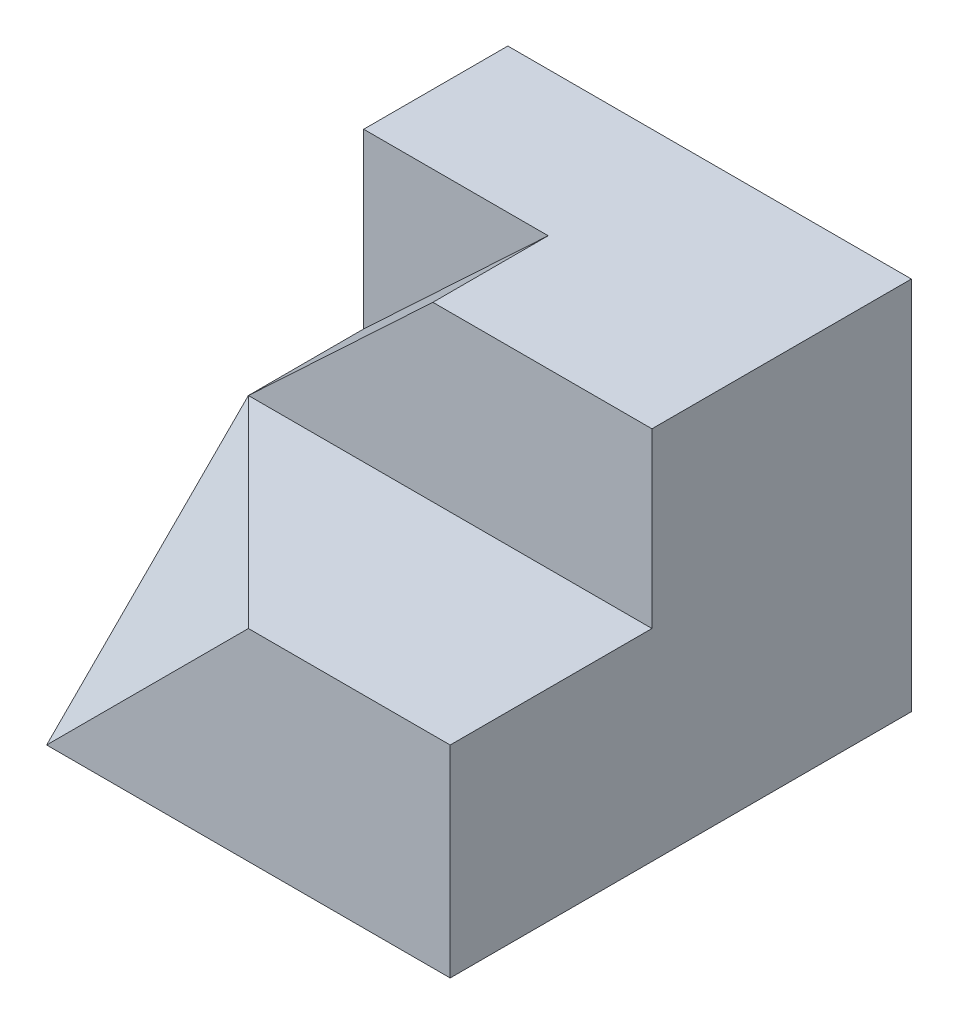
ISO-10303-21;
HEADER;
FILE_DESCRIPTION(('STEP AP214'),'2;1');
FILE_NAME('part.step','',(''),(''),'','','');
FILE_SCHEMA(('AUTOMOTIVE_DESIGN { 1 0 10303 214 1 1 1 1 }'));
ENDSEC;
DATA;
#1=APPLICATION_CONTEXT('core data for automotive mechanical design processes');
#2=APPLICATION_PROTOCOL_DEFINITION('international standard','automotive_design',2000,#1);
#3=PRODUCT_CONTEXT('',#1,'mechanical');
#4=PRODUCT('Part','Part','',(#3));
#5=PRODUCT_RELATED_PRODUCT_CATEGORY('part','',(#4));
#6=PRODUCT_DEFINITION_FORMATION('','',#4);
#7=PRODUCT_DEFINITION_CONTEXT('part definition',#1,'design');
#8=PRODUCT_DEFINITION('design','',#6,#7);
#9=PRODUCT_DEFINITION_SHAPE('','',#8);
#10=(LENGTH_UNIT() NAMED_UNIT(*) SI_UNIT(.MILLI.,.METRE.));
#11=(NAMED_UNIT(*) PLANE_ANGLE_UNIT() SI_UNIT($,.RADIAN.));
#12=(NAMED_UNIT(*) SI_UNIT($,.STERADIAN.) SOLID_ANGLE_UNIT());
#13=UNCERTAINTY_MEASURE_WITH_UNIT(LENGTH_MEASURE(1.E-05),#10,'distance_accuracy_value','');
#14=(GEOMETRIC_REPRESENTATION_CONTEXT(3) GLOBAL_UNCERTAINTY_ASSIGNED_CONTEXT((#13)) GLOBAL_UNIT_ASSIGNED_CONTEXT((#10,
#11,#12)) REPRESENTATION_CONTEXT('',''));
#15=CARTESIAN_POINT('',(0.,0.,0.));
#16=DIRECTION('',(0.,0.,1.));
#17=DIRECTION('',(1.,0.,0.));
#18=AXIS2_PLACEMENT_3D('',#15,#16,#17);
#19=CARTESIAN_POINT('',(0.,65.,40.));
#20=DIRECTION('',(1.,0.,0.));
#21=DIRECTION('',(0.,0.,-1.));
#22=AXIS2_PLACEMENT_3D('',#19,#20,#21);
#23=PLANE('',#22);
#24=DIRECTION('',(0.,0.707106781186548,-0.707106781186548));
#25=VECTOR('',#24,1.);
#26=CARTESIAN_POINT('',(0.,35.,5.));
#27=LINE('',#26,#25);
#28=CARTESIAN_POINT('',(0.,0.,40.));
#29=VERTEX_POINT('',#28);
#30=CARTESIAN_POINT('',(0.,35.,5.));
#31=VERTEX_POINT('',#30);
#32=EDGE_CURVE('E132',#29,#31,#27,.T.);
#33=ORIENTED_EDGE('',*,*,#32,.T.);
#34=DIRECTION('',(0.,0.,1.));
#35=VECTOR('',#34,1.);
#36=CARTESIAN_POINT('',(0.,35.,-15.));
#37=LINE('',#36,#35);
#38=CARTESIAN_POINT('',(0.,35.,-15.));
#39=VERTEX_POINT('',#38);
#40=EDGE_CURVE('E249',#39,#31,#37,.T.);
#41=ORIENTED_EDGE('',*,*,#40,.F.);
#42=DIRECTION('',(0.,-1.,0.));
#43=VECTOR('',#42,1.);
#44=CARTESIAN_POINT('',(0.,65.,-15.));
#45=LINE('',#44,#43);
#46=CARTESIAN_POINT('',(0.,65.,-15.));
#47=VERTEX_POINT('',#46);
#48=EDGE_CURVE('E238',#47,#39,#45,.T.);
#49=ORIENTED_EDGE('',*,*,#48,.F.);
#50=DIRECTION('',(0.,0.,-1.));
#51=VECTOR('',#50,1.);
#52=CARTESIAN_POINT('',(0.,65.,40.));
#53=LINE('',#52,#51);
#54=CARTESIAN_POINT('',(0.,65.,-40.));
#55=VERTEX_POINT('',#54);
#56=EDGE_CURVE('E99',#47,#55,#53,.T.);
#57=ORIENTED_EDGE('',*,*,#56,.T.);
#58=DIRECTION('',(0.,-1.,0.));
#59=VECTOR('',#58,1.);
#60=CARTESIAN_POINT('',(0.,65.,-40.));
#61=LINE('',#60,#59);
#62=CARTESIAN_POINT('',(0.,0.,-40.));
#63=VERTEX_POINT('',#62);
#64=EDGE_CURVE('E115',#55,#63,#61,.T.);
#65=ORIENTED_EDGE('',*,*,#64,.T.);
#66=DIRECTION('',(0.,0.,-1.));
#67=VECTOR('',#66,1.);
#68=CARTESIAN_POINT('',(0.,0.,40.));
#69=LINE('',#68,#67);
#70=EDGE_CURVE('E11',#29,#63,#69,.T.);
#71=ORIENTED_EDGE('',*,*,#70,.F.);
#72=EDGE_LOOP('',(#33,#41,#49,#57,#65,#71));
#73=FACE_BOUND('',#72,.T.);
#74=ADVANCED_FACE('F44',(#73),#23,.F.);
#75=CARTESIAN_POINT('',(0.,0.,40.));
#76=DIRECTION('',(0.,0.,1.));
#77=DIRECTION('',(1.,0.,0.));
#78=AXIS2_PLACEMENT_3D('',#75,#76,#77);
#79=PLANE('',#78);
#80=DIRECTION('',(1.,0.,0.));
#81=VECTOR('',#80,1.);
#82=CARTESIAN_POINT('',(0.,35.,40.));
#83=LINE('',#82,#81);
#84=CARTESIAN_POINT('',(35.,35.,40.));
#85=VERTEX_POINT('',#84);
#86=CARTESIAN_POINT('',(70.,35.,40.));
#87=VERTEX_POINT('',#86);
#88=EDGE_CURVE('E254',#85,#87,#83,.T.);
#89=ORIENTED_EDGE('',*,*,#88,.F.);
#90=DIRECTION('',(-0.707106781186548,-0.707106781186548,0.));
#91=VECTOR('',#90,1.);
#92=CARTESIAN_POINT('',(0.,0.,40.));
#93=LINE('',#92,#91);
#94=EDGE_CURVE('E56',#85,#29,#93,.T.);
#95=ORIENTED_EDGE('',*,*,#94,.T.);
#96=DIRECTION('',(1.,0.,0.));
#97=VECTOR('',#96,1.);
#98=CARTESIAN_POINT('',(0.,0.,40.));
#99=LINE('',#98,#97);
#100=CARTESIAN_POINT('',(70.,0.,40.));
#101=VERTEX_POINT('',#100);
#102=EDGE_CURVE('E70',#29,#101,#99,.T.);
#103=ORIENTED_EDGE('',*,*,#102,.T.);
#104=DIRECTION('',(0.,1.,0.));
#105=VECTOR('',#104,1.);
#106=CARTESIAN_POINT('',(70.,0.,40.));
#107=LINE('',#106,#105);
#108=EDGE_CURVE('E111',#101,#87,#107,.T.);
#109=ORIENTED_EDGE('',*,*,#108,.T.);
#110=EDGE_LOOP('',(#89,#95,#103,#109));
#111=FACE_BOUND('',#110,.T.);
#112=ADVANCED_FACE('F135',(#111),#79,.T.);
#113=CARTESIAN_POINT('',(0.,35.,5.));
#114=DIRECTION('',(0.,-1.,0.));
#115=DIRECTION('',(0.,0.,-1.));
#116=AXIS2_PLACEMENT_3D('',#113,#114,#115);
#117=PLANE('',#116);
#118=DIRECTION('',(0.707106781186548,0.,0.707106781186548));
#119=VECTOR('',#118,1.);
#120=CARTESIAN_POINT('',(35.,35.,40.));
#121=LINE('',#120,#119);
#122=EDGE_CURVE('E276',#31,#85,#121,.T.);
#123=ORIENTED_EDGE('',*,*,#122,.T.);
#124=ORIENTED_EDGE('',*,*,#88,.T.);
#125=DIRECTION('',(0.,0.,1.));
#126=VECTOR('',#125,1.);
#127=CARTESIAN_POINT('',(70.,35.,5.));
#128=LINE('',#127,#126);
#129=CARTESIAN_POINT('',(70.,35.,5.));
#130=VERTEX_POINT('',#129);
#131=EDGE_CURVE('E122',#130,#87,#128,.T.);
#132=ORIENTED_EDGE('',*,*,#131,.F.);
#133=DIRECTION('',(1.,0.,0.));
#134=VECTOR('',#133,1.);
#135=CARTESIAN_POINT('',(0.,35.,5.));
#136=LINE('',#135,#134);
#137=EDGE_CURVE('E257',#31,#130,#136,.T.);
#138=ORIENTED_EDGE('',*,*,#137,.F.);
#139=EDGE_LOOP('',(#123,#124,#132,#138));
#140=FACE_BOUND('',#139,.T.);
#141=ADVANCED_FACE('F139',(#140),#117,.F.);
#142=CARTESIAN_POINT('',(70.,65.,40.));
#143=DIRECTION('',(0.,-1.,0.));
#144=DIRECTION('',(1.,0.,0.));
#145=AXIS2_PLACEMENT_3D('',#142,#143,#144);
#146=PLANE('',#145);
#147=DIRECTION('',(-1.,0.,0.));
#148=VECTOR('',#147,1.);
#149=CARTESIAN_POINT('',(32.,65.,-15.));
#150=LINE('',#149,#148);
#151=CARTESIAN_POINT('',(32.,65.,-15.));
#152=VERTEX_POINT('',#151);
#153=EDGE_CURVE('E245',#152,#47,#150,.T.);
#154=ORIENTED_EDGE('',*,*,#153,.F.);
#155=DIRECTION('',(0.,0.,1.));
#156=VECTOR('',#155,1.);
#157=CARTESIAN_POINT('',(32.,65.,-15.));
#158=LINE('',#157,#156);
#159=CARTESIAN_POINT('',(32.,65.,5.));
#160=VERTEX_POINT('',#159);
#161=EDGE_CURVE('E251',#152,#160,#158,.T.);
#162=ORIENTED_EDGE('',*,*,#161,.T.);
#163=DIRECTION('',(-1.,0.,0.));
#164=VECTOR('',#163,1.);
#165=CARTESIAN_POINT('',(70.,65.,5.));
#166=LINE('',#165,#164);
#167=CARTESIAN_POINT('',(70.,65.,5.));
#168=VERTEX_POINT('',#167);
#169=EDGE_CURVE('E100',#168,#160,#166,.T.);
#170=ORIENTED_EDGE('',*,*,#169,.F.);
#171=DIRECTION('',(0.,0.,-1.));
#172=VECTOR('',#171,1.);
#173=CARTESIAN_POINT('',(70.,65.,40.));
#174=LINE('',#173,#172);
#175=CARTESIAN_POINT('',(70.,65.,-40.));
#176=VERTEX_POINT('',#175);
#177=EDGE_CURVE('E87',#168,#176,#174,.T.);
#178=ORIENTED_EDGE('',*,*,#177,.T.);
#179=DIRECTION('',(-1.,0.,0.));
#180=VECTOR('',#179,1.);
#181=CARTESIAN_POINT('',(70.,65.,-40.));
#182=LINE('',#181,#180);
#183=EDGE_CURVE('E91',#176,#55,#182,.T.);
#184=ORIENTED_EDGE('',*,*,#183,.T.);
#185=ORIENTED_EDGE('',*,*,#56,.F.);
#186=EDGE_LOOP('',(#154,#162,#170,#178,#184,#185));
#187=FACE_BOUND('',#186,.T.);
#188=ADVANCED_FACE('F89',(#187),#146,.F.);
#189=CARTESIAN_POINT('',(0.,0.,40.));
#190=DIRECTION('',(0.,1.,0.));
#191=DIRECTION('',(0.,0.,1.));
#192=AXIS2_PLACEMENT_3D('',#189,#190,#191);
#193=PLANE('',#192);
#194=DIRECTION('',(1.,0.,0.));
#195=VECTOR('',#194,1.);
#196=CARTESIAN_POINT('',(0.,0.,-40.));
#197=LINE('',#196,#195);
#198=CARTESIAN_POINT('',(70.,0.,-40.));
#199=VERTEX_POINT('',#198);
#200=EDGE_CURVE('E107',#63,#199,#197,.T.);
#201=ORIENTED_EDGE('',*,*,#200,.T.);
#202=DIRECTION('',(0.,0.,-1.));
#203=VECTOR('',#202,1.);
#204=CARTESIAN_POINT('',(70.,0.,40.));
#205=LINE('',#204,#203);
#206=EDGE_CURVE('E55',#101,#199,#205,.T.);
#207=ORIENTED_EDGE('',*,*,#206,.F.);
#208=ORIENTED_EDGE('',*,*,#102,.F.);
#209=ORIENTED_EDGE('',*,*,#70,.T.);
#210=EDGE_LOOP('',(#201,#207,#208,#209));
#211=FACE_BOUND('',#210,.T.);
#212=ADVANCED_FACE('F127',(#211),#193,.F.);
#213=CARTESIAN_POINT('',(70.,0.,40.));
#214=DIRECTION('',(-1.,0.,0.));
#215=DIRECTION('',(0.,0.,1.));
#216=AXIS2_PLACEMENT_3D('',#213,#214,#215);
#217=PLANE('',#216);
#218=DIRECTION('',(0.,1.,0.));
#219=VECTOR('',#218,1.);
#220=CARTESIAN_POINT('',(70.,35.,5.));
#221=LINE('',#220,#219);
#222=EDGE_CURVE('E263',#130,#168,#221,.T.);
#223=ORIENTED_EDGE('',*,*,#222,.F.);
#224=ORIENTED_EDGE('',*,*,#131,.T.);
#225=ORIENTED_EDGE('',*,*,#108,.F.);
#226=ORIENTED_EDGE('',*,*,#206,.T.);
#227=DIRECTION('',(0.,1.,0.));
#228=VECTOR('',#227,1.);
#229=CARTESIAN_POINT('',(70.,0.,-40.));
#230=LINE('',#229,#228);
#231=EDGE_CURVE('E102',#199,#176,#230,.T.);
#232=ORIENTED_EDGE('',*,*,#231,.T.);
#233=ORIENTED_EDGE('',*,*,#177,.F.);
#234=EDGE_LOOP('',(#223,#224,#225,#226,#232,#233));
#235=FACE_BOUND('',#234,.T.);
#236=ADVANCED_FACE('F104',(#235),#217,.F.);
#237=CARTESIAN_POINT('',(0.,0.,-40.));
#238=DIRECTION('',(0.,0.,1.));
#239=DIRECTION('',(1.,0.,0.));
#240=AXIS2_PLACEMENT_3D('',#237,#238,#239);
#241=PLANE('',#240);
#242=ORIENTED_EDGE('',*,*,#64,.F.);
#243=ORIENTED_EDGE('',*,*,#183,.F.);
#244=ORIENTED_EDGE('',*,*,#231,.F.);
#245=ORIENTED_EDGE('',*,*,#200,.F.);
#246=EDGE_LOOP('',(#242,#243,#244,#245));
#247=FACE_BOUND('',#246,.T.);
#248=ADVANCED_FACE('F109',(#247),#241,.F.);
#249=CARTESIAN_POINT('',(0.,0.,5.));
#250=DIRECTION('',(0.,0.,1.));
#251=DIRECTION('',(1.,0.,0.));
#252=AXIS2_PLACEMENT_3D('',#249,#250,#251);
#253=PLANE('',#252);
#254=DIRECTION('',(0.729537204140085,0.68394112888133,0.));
#255=VECTOR('',#254,1.);
#256=CARTESIAN_POINT('',(0.,35.,5.));
#257=LINE('',#256,#255);
#258=EDGE_CURVE('E248',#31,#160,#257,.T.);
#259=ORIENTED_EDGE('',*,*,#258,.F.);
#260=ORIENTED_EDGE('',*,*,#137,.T.);
#261=ORIENTED_EDGE('',*,*,#222,.T.);
#262=ORIENTED_EDGE('',*,*,#169,.T.);
#263=EDGE_LOOP('',(#259,#260,#261,#262));
#264=FACE_BOUND('',#263,.T.);
#265=ADVANCED_FACE('F151',(#264),#253,.T.);
#266=CARTESIAN_POINT('',(0.,35.,-15.));
#267=DIRECTION('',(0.68394112888133,-0.729537204140085,0.));
#268=DIRECTION('',(0.729537204140085,0.68394112888133,0.));
#269=AXIS2_PLACEMENT_3D('',#266,#267,#268);
#270=PLANE('',#269);
#271=ORIENTED_EDGE('',*,*,#258,.T.);
#272=ORIENTED_EDGE('',*,*,#161,.F.);
#273=DIRECTION('',(0.729537204140085,0.68394112888133,0.));
#274=VECTOR('',#273,1.);
#275=CARTESIAN_POINT('',(0.,35.,-15.));
#276=LINE('',#275,#274);
#277=EDGE_CURVE('E244',#39,#152,#276,.T.);
#278=ORIENTED_EDGE('',*,*,#277,.F.);
#279=ORIENTED_EDGE('',*,*,#40,.T.);
#280=EDGE_LOOP('',(#271,#272,#278,#279));
#281=FACE_BOUND('',#280,.T.);
#282=ADVANCED_FACE('F169',(#281),#270,.F.);
#283=CARTESIAN_POINT('',(0.,0.,-15.));
#284=DIRECTION('',(0.,0.,-1.));
#285=DIRECTION('',(-1.,0.,0.));
#286=AXIS2_PLACEMENT_3D('',#283,#284,#285);
#287=PLANE('',#286);
#288=ORIENTED_EDGE('',*,*,#48,.T.);
#289=ORIENTED_EDGE('',*,*,#277,.T.);
#290=ORIENTED_EDGE('',*,*,#153,.T.);
#291=EDGE_LOOP('',(#288,#289,#290));
#292=FACE_BOUND('',#291,.T.);
#293=ADVANCED_FACE('F180',(#292),#287,.F.);
#294=CARTESIAN_POINT('',(-13.3333333333333,13.3333333333333,13.3333333333333));
#295=DIRECTION('',(-0.577350269189626,0.577350269189626,0.577350269189626));
#296=DIRECTION('',(0.,-0.707106781186548,0.707106781186547));
#297=AXIS2_PLACEMENT_3D('',#294,#295,#296);
#298=PLANE('',#297);
#299=ORIENTED_EDGE('',*,*,#122,.F.);
#300=ORIENTED_EDGE('',*,*,#32,.F.);
#301=ORIENTED_EDGE('',*,*,#94,.F.);
#302=EDGE_LOOP('',(#299,#300,#301));
#303=FACE_BOUND('',#302,.T.);
#304=ADVANCED_FACE('F184',(#303),#298,.T.);
#305=CLOSED_SHELL('',(#74,#112,#141,#188,#212,#236,#248,#265,#282,#293,#304));
#306=MANIFOLD_SOLID_BREP('B2',#305);
#307=ADVANCED_BREP_SHAPE_REPRESENTATION('',(#18,#306),#14);
#308=SHAPE_DEFINITION_REPRESENTATION(#9,#307);
ENDSEC;
END-ISO-10303-21;
